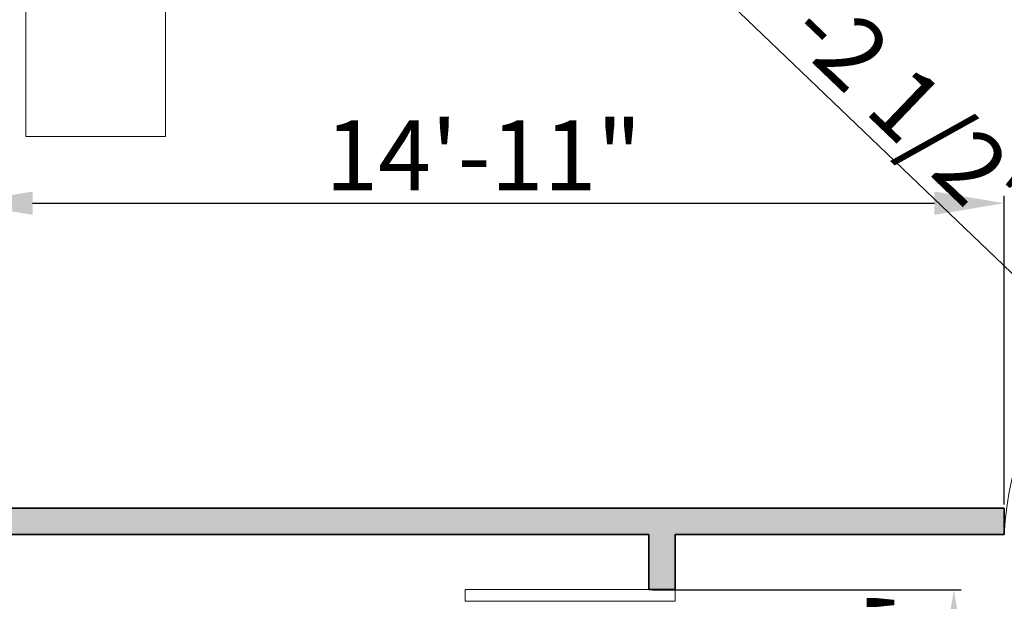
# Model space of a CAD drawing. Units: inches. Extents: x 2083 to 3317, y 1141 to 2115.
# Tile 93 of 256: x 2246 to 2415, y 1794 to 1894. Entities that reach past the tile are written whole.
import ezdxf

# ---------------------------------------------------------------- set-up
doc = ezdxf.new("R2010")
doc.units = ezdxf.units.IN
for name, color, linetype, lineweight in [('A-ANNO-DIMS', 2, 'Continuous', 18), ('A-DOOR', 4, 'Continuous', 18), ('A-FURN', 8, 'Continuous', 18), ('A-WALL', 7, 'Continuous', 35)]:
    doc.layers.add(name, color=color, linetype=linetype, lineweight=lineweight)
doc.layers.add('A-WALL-PATT', color=251, linetype='Continuous', lineweight=13, true_color=0x636466)
doc.styles.get("Standard").update_dxf_attribs({"font": 'arial.ttf'})
doc.dimstyles.new('ISO-25', dxfattribs={"dimtxt": 12, "dimasz": 12, "dimexe": 1.25, "dimexo": 0.625, "dimtad": 1, "dimlunit": 3, "dimtxsty": 'Standard', "dimcen": 2.5, "dimadec": 0, "dimazin": 0, "dimtfac": 1, "dimtmove": 0, "dimatfit": 3, "dimfxl": 1, "dimarcsym": 0})

# ---------------------------------------------------------------- blocks, each defined once
blk = doc.blocks.new('*D53')
at = {"layer": 'A-ANNO-DIMS', "color": 0, "lineweight": -2, "transparency": 16777216}
for p, q in [((2235.96, 1810.64), (2235.96, 1863.61)), ((2247.96, 1862.36), (2402.72, 1862.36)), ((2414.72, 1810.64), (2414.72, 1863.61))]:
    blk.add_line(p, q, dxfattribs=at)
at = {"layer": 'A-ANNO-DIMS', "color": 0, "transparency": 16777216}
for points in [[(2247.96, 1864.36), (2247.96, 1860.36), (2235.96, 1862.36)], [(2402.72, 1864.36), (2402.72, 1860.36), (2414.72, 1862.36)]]:
    blk.add_solid(points, dxfattribs=at)
at = {"layer": 'Defpoints', "color": 0, "transparency": 16777216}
for p in [(2414.72, 1862.36), (2235.96, 1810.01), (2414.72, 1810.01)]:
    blk.add_point(p, dxfattribs=at)
at = {"layer": 'A-ANNO-DIMS', "color": 0, "transparency": 16777216, "insert": (2325.34, 1869.01), "char_height": 12, "attachment_point": 5}
blk.add_mtext('14\'-11"', dxfattribs=at)
blk = doc.blocks.new('*D56')
at = {"layer": 'A-ANNO-DIMS', "color": 0, "lineweight": -2, "transparency": 16777216}
for p, q in [((2354.33, 1796.05), (2407.31, 1796.05)), ((2406.06, 1784.05), (2406.06, 1772.05)), ((2354.33, 1760.05), (2407.31, 1760.05))]:
    blk.add_line(p, q, dxfattribs=at)
at = {"layer": 'A-ANNO-DIMS', "color": 0, "transparency": 16777216}
for points in [[(2404.06, 1784.05), (2408.06, 1784.05), (2406.06, 1796.05)], [(2404.06, 1772.05), (2408.06, 1772.05), (2406.06, 1760.05)]]:
    blk.add_solid(points, dxfattribs=at)
at = {"layer": 'Defpoints', "color": 0, "transparency": 16777216}
for p in [(2353.71, 1796.05), (2353.71, 1760.05), (2406.06, 1760.05)]:
    blk.add_point(p, dxfattribs=at)
at = {"layer": 'A-ANNO-DIMS', "color": 0, "transparency": 16777216, "insert": (2399.3, 1778.05), "char_height": 12, "attachment_point": 5, "rotation": 90}
blk.add_mtext('3\'-0"', dxfattribs=at)
blk = doc.blocks.new('*D68')
at = {"layer": 'A-ANNO-DIMS', "color": 0, "lineweight": -2, "transparency": 16777216}
for p, q in [((2358.93, 1905.02), (2420.01, 1846.48)), ((2465.03, 1803.34), (2428.67, 1838.18))]:
    blk.add_line(p, q, dxfattribs=at)
at = {"layer": 'A-ANNO-DIMS', "color": 0, "transparency": 16777216}
blk.add_solid([(2421.39, 1847.93), (2418.62, 1845.04), (2428.67, 1838.18)], dxfattribs=at)
at = {"layer": 'Defpoints', "color": 0, "transparency": 16777216}
for p in [(2428.67, 1838.18), (2465.03, 1803.34)]:
    blk.add_point(p, dxfattribs=at)
at = {"layer": 'A-ANNO-DIMS', "color": 0, "transparency": 16777216, "insert": (2389.86, 1884.83), "char_height": 12, "attachment_point": 5, "rotation": 316.2184}
blk.add_mtext('R4\'-2 1/2"', dxfattribs=at)

msp = doc.modelspace()

# ---------------------------------------------------------------- hatches: boundary and pattern name
at = {"layer": 'A-WALL-PATT'}
h = msp.add_hatch(color=256, dxfattribs=at)
h.dxf.hatch_style = 1
h.paths.add_polyline_path([(3126.96, 2020.761), (2748.96, 2020.761), (2604.96, 2020.761), (2226.96, 2020.761), (2226.96, 1702.761), (2466.96, 1702.761), (2466.96, 1582.761), (2418.96, 1582.761), (2418.96, 1477.761), (2226.96, 1477.761), (2226.96, 1263.261), (2544.96, 1263.261), (2544.96, 1411.761), (2604.96, 1411.761), (2685.96, 1411.761), (2685.96, 1420.761), (2604.96, 1420.761), (2604.96, 1573.761), (2604.96, 1702.761), (2604.96, 2011.761), (2748.96, 2011.761), (2748.96, 1702.761), (2862.96, 1702.761), (2862.96, 1621.761), (2871.96, 1621.761), (2871.96, 1702.761), (2883.96, 1702.761), (2883.96, 1706.939, -0.0264593), (2883.96, 1711.761), (2757.96, 1711.761), (2757.96, 1807.761), (2787.96, 1807.761), (2787.96, 1812.261), (2757.96, 1812.261), (2757.96, 2011.761), (2877.96, 2011.761), (2877.96, 1812.261), (2847.96, 1812.261), (2847.96, 1807.761), (2889.836, 1807.761), (2889.836, 1812.261), (2882.46, 1812.261), (2882.46, 2011.761), (3117.96, 2011.761), (3117.96, 1812.261), (2937.836, 1812.261), (2937.836, 1807.761), (2995.71, 1807.761), (2995.71, 1796.118), (3000.21, 1796.118), (3000.21, 1807.761), (3117.96, 1807.761), (3117.96, 1711.761), (3000.21, 1711.761), (3000.21, 1760.118), (2998.573, 1760.118, -0.020711), (2995.71, 1760.118), (2995.71, 1711.761), (2931.96, 1711.761), (2931.96, 1702.761), (3126.96, 1702.761)])
h.paths.add_polyline_path([(2471.46, 2011.761), (2471.46, 1810.011), (2462.717, 1810.011), (2462.717, 1805.511), (2505.96, 1805.511), (2505.96, 1810.011), (2475.96, 1810.011), (2475.96, 2011.761), (2595.96, 2011.761), (2595.96, 1810.011), (2565.96, 1810.011), (2565.96, 1805.511), (2595.96, 1805.511), (2595.96, 1711.761), (2235.96, 1711.761), (2235.96, 1805.511), (2353.71, 1805.511), (2353.71, 1796.054), (2358.21, 1796.054), (2358.21, 1805.511), (2414.717, 1805.511), (2414.717, 1810.011), (2235.96, 1810.011), (2235.96, 2011.761)], flags=16)
h.paths.add_polyline_path([(2270.205, 1994.61), (2270.205, 1970.61), (2246.205, 1970.61), (2246.205, 1994.61)], flags=0)
edge = h.paths.add_edge_path(flags=0)
edge.add_ellipse((2332.027, 1899.798), major_axis=(-3.043, 3.043), ratio=0.1682525, start_angle=-161.33217, end_angle=-156.30711, ccw=False)
edge.add_ellipse((2333.082, 1898.744), major_axis=(-1.055, 1.055), ratio=0.4535321, start_angle=-123.37102, end_angle=-94.15911)
edge = h.paths.add_edge_path(flags=0)
edge.add_ellipse((2332.027, 1968.876), major_axis=(3.043, 3.043), ratio=0.1682525, start_angle=18.66783, end_angle=23.69289)
edge.add_spline(control_points=[(2332.926, 1970.691), (2332.227, 1970.336), (2330.894, 1969.659), (2328.413, 1970.932), (2327.204, 1967.749), (2324.71, 1969.956), (2322.533, 1967.012), (2320.013, 1971.296), (2317.68, 1968.158), (2316.041, 1967.102), (2315.427, 1966.81)], knot_values=[0, 0, 0, 0, 2.2670587, 4.3245589, 6.6855835, 8.8786411, 11.121502, 14.300359, 17.7552837, 19.732645, 19.732645, 19.732645, 19.732645], degree=3, periodic=0)
edge.add_ellipse((2332.027, 1968.876), major_axis=(3.043, 3.043), ratio=0.1682525, start_angle=18.66783, end_angle=23.69289, ccw=False)
edge.add_ellipse((2333.082, 1969.931), major_axis=(1.055, 1.055), ratio=0.4535321, start_angle=56.62898, end_angle=85.84089, ccw=False)
edge = h.paths.add_edge_path(flags=0)
edge.add_spline(control_points=[(2296.428, 1967.988), (2293.628, 1965.336), (2287.704, 1959.727), (2299.744, 1949.996), (2294.533, 1935.669), (2290.573, 1920.604), (2293.394, 1909.974), (2296.185, 1904.967)], knot_values=[0.0991853, 0.0991853, 0.0991853, 0.0991853, 0.3453009, 0.6198217, 0.9826526, 1.3860932, 1.8105546, 1.8105546, 1.8105546, 1.8105546], degree=3, periodic=0)
edge.add_spline(control_points=[(2296.185, 1904.967), (2297.384, 1902.619), (2298.001, 1901.949), (2298.553, 1901.468)], knot_values=[0.0062457, 0.0062457, 0.0062457, 0.0062457, 0.0554759, 0.0554759, 0.0554759, 0.0554759], degree=3, periodic=0)
edge.add_spline(control_points=[(2298.553, 1901.468), (2297.259, 1900.923), (2295.225, 1900.232), (2293.06, 1900.614), (2292.101, 1900.788), (2292.09, 1900.791)], knot_values=[0.3128349, 0.3128349, 0.3128349, 0.3128349, 0.4017797, 0.4749867, 0.4759027, 0.4759027, 0.4759027, 0.4759027], degree=3, periodic=0)
edge.add_arc((2292.794, 1904.664), 3.937, 215.4209, 259.69818, ccw=False)
edge.add_spline(control_points=[(2289.585, 1902.382), (2289.477, 1902.535), (2289.368, 1902.688), (2289.261, 1902.841)], knot_values=[0.1028719, 0.1028719, 0.1028719, 0.1028719, 0.1168958, 0.1168958, 0.1168958, 0.1168958], degree=3, periodic=0)
edge.add_spline(control_points=[(2289.261, 1902.841), (2288.687, 1902.55), (2287.64, 1902.02), (2285.881, 1901.874), (2283.853, 1901.504), (2281.72, 1899.711), (2278.467, 1899.493), (2276.157, 1901.883), (2272.259, 1899.804), (2267.778, 1901.843), (2262.244, 1900.184), (2257.415, 1901.782), (2254.318, 1900.726), (2253.178, 1900.337)], knot_values=[0, 0, 0, 0, 1.9079767, 3.4771759, 5.261074, 7.9728515, 11.6802485, 13.7179214, 16.9395917, 22.789562, 27.5025027, 33.5952153, 37.1456181, 37.1456181, 37.1456181, 37.1456181], degree=3, periodic=0)
edge.add_line((2253.178, 1900.337), (2250.244, 1902.841))
edge.add_line((2250.244, 1902.841), (2250.244, 1965.833))
edge.add_line((2250.244, 1965.833), (2253.178, 1968.337))
edge.add_spline(control_points=[(2253.178, 1968.337), (2254.318, 1967.948), (2257.415, 1966.892), (2262.244, 1968.49), (2267.778, 1966.831), (2271.527, 1968.537), (2273.876, 1967.828), (2274.207, 1967.728)], knot_values=[0, 0, 0, 0, 0.0901802, 0.2449351, 0.3646438, 0.5132331, 0.5378548, 0.5378548, 0.5378548, 0.5378548], degree=3, periodic=0)
edge.add_arc((2274.353, 1963.793), 3.937, 72.05113, 92.12795, ccw=False)
edge.add_arc((2281.297, 1985.23), 18.596, 252.05113, 288.56572)
edge.add_arc((2292.317, 1956.029), 12.646, 71.02679, 113.77822, ccw=False)
edge = h.paths.add_edge_path(flags=0)
edge.add_spline(control_points=[(2274.899, 1951.856), (2275.066, 1951.617), (2275.233, 1951.377), (2275.398, 1951.136)], knot_values=[1.4099157, 1.4099157, 1.4099157, 1.4099157, 1.4315903, 1.4315903, 1.4315903, 1.4315903], degree=3, periodic=0)
edge.add_spline(control_points=[(2275.398, 1951.136), (2275.792, 1950.562), (2276.179, 1949.984), (2276.546, 1949.397)], knot_values=[1.3582378, 1.3582378, 1.3582378, 1.3582378, 1.4099157, 1.4099157, 1.4099157, 1.4099157], degree=3, periodic=0)
edge.add_line((2276.546, 1949.397), (2277.437, 1947.862))
edge.add_spline(control_points=[(2277.437, 1947.862), (2276.304, 1945.673), (2274.64, 1942.427), (2274.632, 1938.094), (2272.799, 1930.852), (2274.356, 1943.897), (2275.948, 1947.923), (2276.546, 1949.397)], knot_values=[0.0056315, 0.0056315, 0.0056315, 0.0056315, 0.1860139, 0.2660015, 0.3570872, 0.5963902, 0.7397317, 0.7397317, 0.7397317, 0.7397317], degree=3, periodic=0)
edge.add_spline(control_points=[(2276.546, 1949.397), (2276.179, 1949.984), (2275.792, 1950.562), (2275.398, 1951.136)], knot_values=[1.3582378, 1.3582378, 1.3582378, 1.3582378, 1.4099157, 1.4099157, 1.4099157, 1.4099157], degree=3, periodic=0)
edge.add_spline(control_points=[(2275.398, 1951.136), (2274.943, 1950.08), (2274.208, 1948.025), (2273.935, 1944.851), (2272.469, 1937.627), (2273.466, 1945.696), (2274.701, 1951.059), (2274.899, 1951.856)], knot_values=[0.1043639, 0.1043639, 0.1043639, 0.1043639, 0.1896363, 0.2696239, 0.3607096, 0.6000126, 0.6446217, 0.6446217, 0.6446217, 0.6446217], degree=3, periodic=0)
h.paths.add_polyline_path([(2269.168, 1963.128, -0.3575267), (2268.171, 1960.976, -0.0925607), (2268.171, 1939.436, -0.3575267), (2269.168, 1937.285, -0.3575267), (2267.016, 1938.282, -0.1647847), (2254.686, 1938.282, -0.3575267), (2252.534, 1937.285, -0.3575267), (2253.531, 1939.436, -0.0925607), (2253.531, 1960.976, -0.3575267), (2252.534, 1963.128, -0.3575267), (2254.686, 1962.131, -0.1647847), (2267.016, 1962.131, -0.3575267)], flags=0)
h.paths.add_polyline_path([(2248.874, 1967.802), (2248.874, 1957.028), (2249.458, 1957.028), (2249.458, 1911.647), (2248.874, 1911.647), (2248.874, 1900.873), (2246.512, 1900.873, 0.1973271), (2244.15, 1902.457), (2244.15, 1966.218, 0.1973271), (2246.512, 1967.802)], flags=0)
h.paths.add_polyline_path([(2269.168, 1931.389, -0.3575267), (2268.171, 1929.238, -0.0925607), (2268.171, 1907.698, -0.3575267), (2269.168, 1905.547, -0.3575267), (2267.016, 1906.544, -0.1647847), (2254.686, 1906.544, -0.3575267), (2252.534, 1905.547, -0.3575267), (2253.531, 1907.698, -0.0925607), (2253.531, 1929.238, -0.3575267), (2252.534, 1931.389, -0.3575267), (2254.686, 1930.392, -0.1647847), (2267.016, 1930.392, -0.3575267)], flags=0)
edge = h.paths.add_edge_path(flags=0)
edge.add_spline(control_points=[(2276.197, 1906.724), (2276.168, 1909.029), (2276.114, 1913.372), (2270.598, 1924.925), (2273.905, 1919.013), (2275.922, 1916.262), (2275.475, 1912.402), (2277.258, 1910.381), (2276.696, 1908.225), (2276.646, 1906.813), (2276.618, 1906.008)], knot_values=[0, 0, 0, 0, 8.6102597, 16.2212739, 18.8430575, 23.8048978, 27.4408283, 29.3561016, 31.2034776, 33.6506866, 33.6506866, 33.6506866, 33.6506866], degree=3, periodic=0)
edge.add_spline(control_points=[(2276.618, 1906.008), (2276.623, 1905.624), (2276.498, 1904.629), (2275.442, 1903.855), (2274.937, 1903.08), (2274.859, 1902.841)], knot_values=[0.1564884, 0.1564884, 0.1564884, 0.1564884, 0.1843975, 0.2313765, 0.2505985, 0.2505985, 0.2505985, 0.2505985], degree=3, periodic=0)
edge.add_line((2274.859, 1902.841), (2276.506, 1902.841))
edge.add_spline(control_points=[(2276.506, 1902.841), (2276.788, 1903.085), (2277.665, 1904.125), (2278.25, 1904.341), (2277.654, 1908.527), (2278.156, 1906.228), (2278.1, 1905.286), (2278.847, 1904.069), (2277.857, 1903.415), (2277.874, 1902.991), (2277.904, 1902.841)], knot_values=[0.0595743, 0.0595743, 0.0595743, 0.0595743, 0.0807529, 0.1037415, 0.1697201, 0.1760361, 0.2071372, 0.2404744, 0.2623409, 0.2736605, 0.2736605, 0.2736605, 0.2736605], degree=3, periodic=0)
edge.add_line((2277.904, 1902.841), (2280.03, 1902.841))
edge.add_spline(control_points=[(2280.03, 1902.841), (2279.888, 1903.088), (2279.499, 1903.982), (2280.152, 1905.939), (2278.104, 1909.658), (2279.762, 1907.185), (2280.328, 1904.875), (2280.485, 1903.49), (2281.463, 1903.249), (2281.758, 1902.936), (2281.834, 1902.841)], knot_values=[0.013856, 0.013856, 0.013856, 0.013856, 0.0348738, 0.0888667, 0.1078792, 0.1267378, 0.158714, 0.1937575, 0.2174868, 0.2267221, 0.2267221, 0.2267221, 0.2267221], degree=3, periodic=0)
edge.add_spline(control_points=[(2281.834, 1902.841), (2281.788, 1902.827), (2281.647, 1902.783), (2281.396, 1902.859), (2281.088, 1902.985), (2280.721, 1903.061), (2280.333, 1903.026), (2280.125, 1902.899), (2280.03, 1902.841)], knot_values=[0, 0, 0, 0, 0.1441304, 0.435517, 0.7492759, 1.1530457, 1.5483707, 1.878348, 1.878348, 1.878348, 1.878348], degree=3, periodic=0)
edge.add_line((2280.03, 1902.841), (2277.904, 1902.841))
edge.add_spline(control_points=[(2277.904, 1902.841), (2277.893, 1902.796), (2277.865, 1902.68), (2277.607, 1902.687), (2277.274, 1902.801), (2276.838, 1902.62), (2276.584, 1902.789), (2276.506, 1902.841)], knot_values=[0, 0, 0, 0, 0.1271885, 0.3261988, 0.6280094, 1.2435704, 1.5153306, 1.5153306, 1.5153306, 1.5153306], degree=3, periodic=0)
edge.add_line((2276.506, 1902.841), (2274.859, 1902.841))
edge.add_spline(control_points=[(2274.859, 1902.841), (2274.814, 1902.899), (2274.725, 1903.013), (2274.493, 1903.119), (2274.244, 1902.961), (2273.937, 1903.185), (2273.614, 1902.983), (2273.408, 1902.883), (2273.322, 1902.841)], knot_values=[0, 0, 0, 0, 0.2184302, 0.4369566, 0.6879766, 0.9903786, 1.3983955, 1.6918498, 1.6918498, 1.6918498, 1.6918498], degree=3, periodic=0)
edge.add_spline(control_points=[(2273.322, 1902.841), (2273.617, 1903.446), (2274.274, 1904.538), (2276.027, 1904.574), (2276.207, 1906.584), (2276.197, 1906.724)], knot_values=[0.0122268, 0.0122268, 0.0122268, 0.0122268, 0.0594721, 0.1062177, 0.134458, 0.134458, 0.134458, 0.134458], degree=3, periodic=0)
h.paths.add_polyline_path([(2270.776, 1897.79), (2270.776, 1873.79), (2246.776, 1873.79), (2246.776, 1897.79)], flags=0)
h.paths.add_polyline_path([(2353.71, 1760.005), (2353.71, 1760.054), (2358.21, 1760.054, -0.033729)], flags=0)
h.paths.add_polyline_path([(2321.819, 1737.529), (2341.995, 1737.529, -0.4142136), (2343.203, 1736.321), (2343.203, 1721.021, -0.4142136), (2341.995, 1719.813), (2321.819, 1719.813, -0.4142136), (2320.611, 1721.021), (2320.611, 1736.321, -0.4142136)], flags=0)
h.paths.add_polyline_path([(2324.235, 1736.321), (2339.579, 1736.321, -0.4142136), (2341.995, 1733.905), (2341.995, 1725.45, -0.4142136), (2339.579, 1723.034), (2333.681, 1723.034), (2333.845, 1722.045, -0.8706461), (2335.425, 1721.826, -0.767327), (2333.923, 1721.423), (2331.291, 1721.423, -0.767327), (2329.788, 1721.826, -0.8706461), (2331.368, 1722.045), (2331.533, 1723.034), (2324.235, 1723.034, -0.4142136), (2321.819, 1725.45), (2321.819, 1733.905, -0.4142136)], flags=0)
h.paths.add_polyline_path([(2570.484, 1928.615), (2589.684, 1928.615), (2590.169, 1928.615), (2590.169, 1904.993), (2570.484, 1904.993)], flags=0)
h.paths.add_polyline_path([(2574.447, 1927.264, -1), (2572.829, 1927.264, -1)], flags=0)
h.paths.add_polyline_path([(2573.09, 1926.941), (2573.925, 1927.776), (2574.148, 1927.553), (2573.313, 1926.718)], flags=0)
h.paths.add_polyline_path([(2578.779, 1919.73, -1), (2571.592, 1919.73, -1)], flags=0)
h.paths.add_polyline_path([(2578.385, 1919.73, -1), (2571.985, 1919.73, -1)], flags=0)
h.paths.add_polyline_path([(2331.596, 1729.476, -1), (2333.618, 1729.476, -1)], flags=0)
h.paths.add_polyline_path([(2578.034, 1927.264, -1), (2576.416, 1927.264, -1)], flags=0)
h.paths.add_polyline_path([(2576.689, 1927.531), (2576.912, 1927.754), (2577.747, 1926.919), (2577.524, 1926.696)], flags=0)
h.paths.add_polyline_path([(2578.139, 1909.86, -1), (2572.232, 1909.86, -1)], flags=0)
h.paths.add_polyline_path([(2577.745, 1909.86, -1), (2572.625, 1909.86, -1)], flags=0)
h.paths.add_polyline_path([(2583.798, 1927.264, -1), (2582.179, 1927.264, -1)], flags=0)
h.paths.add_polyline_path([(2582.719, 1927.754), (2583.554, 1926.919), (2583.331, 1926.696), (2582.496, 1927.531)], flags=0)
h.paths.add_polyline_path([(2582.496, 1927.531), (2582.719, 1927.754), (2583.554, 1926.919), (2583.331, 1926.696)], flags=0)
h.paths.add_polyline_path([(2587.739, 1920.53, -1), (2581.832, 1920.53, -1)], flags=0)
h.paths.add_polyline_path([(2587.345, 1920.53, -1), (2582.225, 1920.53, -1)], flags=0)
h.paths.add_polyline_path([(2587.385, 1927.264, -1), (2585.766, 1927.264, -1)], flags=0)
h.paths.add_polyline_path([(2586.082, 1926.98), (2586.917, 1927.815), (2587.14, 1927.593), (2586.305, 1926.758)], flags=0)
h.paths.add_polyline_path([(2588.379, 1910.66, -1), (2581.192, 1910.66, -1)], flags=0)
h.paths.add_polyline_path([(2587.985, 1910.66, -1), (2581.585, 1910.66, -1)], flags=0)
h.paths.add_polyline_path([(2417.168, 1729.478), (2437.344, 1729.478, -0.4142136), (2438.552, 1728.27), (2438.552, 1712.969, -0.4142136), (2437.344, 1711.761), (2417.168, 1711.761, -0.4142136), (2415.96, 1712.969), (2415.96, 1728.27, -0.4142136)], flags=0)
h.paths.add_polyline_path([(2419.584, 1728.27), (2434.928, 1728.27, -0.4142136), (2437.344, 1725.854), (2437.344, 1717.398, -0.4142136), (2434.928, 1714.983), (2429.029, 1714.983), (2429.194, 1713.994, -0.8706461), (2430.774, 1713.775, -0.767327), (2429.271, 1713.372), (2426.64, 1713.372, -0.767327), (2425.137, 1713.775, -0.8706461), (2426.717, 1713.994), (2426.882, 1714.983), (2419.584, 1714.983, -0.4142136), (2417.168, 1717.398), (2417.168, 1725.854, -0.4142136)], flags=0)
h.paths.add_polyline_path([(2419.584, 1728.27), (2434.928, 1728.27, -0.4142136), (2437.344, 1725.854), (2437.344, 1717.398, -0.4142136), (2434.928, 1714.983), (2429.029, 1714.983), (2428.358, 1719.009), (2427.553, 1719.009), (2426.882, 1714.983), (2419.584, 1714.983, -0.4142136), (2417.168, 1717.398), (2417.168, 1725.854, -0.4142136)], flags=0)
h.paths.add_polyline_path([(2426.944, 1721.425, -1), (2428.967, 1721.425, -1)], flags=0)
h.paths.add_polyline_path([(2475.96, 1702.761), (2595.96, 1702.761), (2595.96, 1582.761), (2475.96, 1582.761)], flags=16)
h.paths.add_polyline_path([(2427.96, 1573.761), (2595.96, 1573.761), (2595.96, 1468.761), (2595.96, 1420.761), (2384.46, 1420.761), (2384.46, 1468.761), (2427.96, 1468.761)], flags=16)
h.paths.add_polyline_path([(2379.96, 1468.761), (2379.96, 1420.761), (2235.96, 1420.761), (2235.96, 1468.761)], flags=16)
h.paths.add_polyline_path([(2317.816, 1466.696), (2337.992, 1466.696, -0.4142136), (2339.2, 1465.488), (2339.2, 1450.187, -0.4142136), (2337.992, 1448.979), (2317.816, 1448.979, -0.4142136), (2316.608, 1450.187), (2316.608, 1465.488, -0.4142136)], flags=0)
h.paths.add_polyline_path([(2320.232, 1465.488), (2335.576, 1465.488, -0.4142136), (2337.992, 1463.072), (2337.992, 1454.616, -0.4142136), (2335.576, 1452.2), (2329.677, 1452.2), (2329.842, 1451.212, -0.8706461), (2331.422, 1450.992, -0.767327), (2329.92, 1450.59), (2327.288, 1450.59, -0.767327), (2325.785, 1450.992, -0.8706461), (2327.365, 1451.212), (2327.53, 1452.2), (2320.232, 1452.2, -0.4142136), (2317.816, 1454.616), (2317.816, 1463.072, -0.4142136)], flags=0)
h.paths.add_polyline_path([(2320.232, 1465.488), (2335.576, 1465.488, -0.4142136), (2337.992, 1463.072), (2337.992, 1454.616, -0.4142136), (2335.576, 1452.2), (2329.677, 1452.2), (2329.006, 1456.227), (2328.201, 1456.227), (2327.53, 1452.2), (2320.232, 1452.2, -0.4142136), (2317.816, 1454.616), (2317.816, 1463.072, -0.4142136)], flags=0)
h.paths.add_polyline_path([(2327.593, 1458.643, -1), (2329.615, 1458.643, -1)], flags=0)
h.paths.add_polyline_path([(2244.412, 1433.34), (2241.921, 1433.34, -0.4142136), (2240.018, 1435.244), (2240.018, 1440.953, -0.4142105), (2241.921, 1442.856), (2244.412, 1442.856, -1.9764724)], flags=0)
h.paths.add_polyline_path([(2245.357, 1434.398, -0.4142136), (2245.357, 1441.799, -2.1440985)], flags=0)
h.paths.add_polyline_path([(2535.96, 1416.261), (2535.96, 1272.261), (2235.96, 1272.261), (2235.96, 1416.261)], flags=16)
h.paths.add_polyline_path([(2260.12, 1384.293), (2260.12, 1362.039), (2237.865, 1362.039), (2237.865, 1384.293)], flags=0)
edge = h.paths.add_edge_path(flags=0)
edge.add_line((2318.252, 1362.093), (2318.146, 1362.001))
edge.add_ellipse((2317.445, 1360.431), major_axis=(2.822, 2.822), ratio=0.1682525, start_angle=18.66783, end_angle=20.94813, ccw=False)
edge.add_ellipse((2318.423, 1361.409), major_axis=(0.978, 0.978), ratio=0.4535321, start_angle=56.62898, end_angle=70.2262, ccw=False)
edge = h.paths.add_edge_path(flags=0)
edge.add_line((2319.107, 1295.571), (2319.015, 1295.677))
edge.add_ellipse((2317.445, 1296.378), major_axis=(-2.822, 2.822), ratio=0.1682525, start_angle=-161.33217, end_angle=-159.05187, ccw=False)
edge.add_ellipse((2318.423, 1295.4), major_axis=(-0.978, 0.978), ratio=0.4535321, start_angle=-123.37102, end_angle=-109.7738)
edge = h.paths.add_edge_path(flags=0)
edge.add_spline(control_points=[(2284.21, 1301.17), (2284.581, 1300.445), (2284.891, 1299.892), (2285.16, 1299.461)], knot_values=[0.0390658, 0.0390658, 0.0390658, 0.0390658, 0.0554759, 0.0554759, 0.0554759, 0.0554759], degree=3, periodic=0)
edge.add_line((2285.16, 1299.461), (2284.21, 1301.17))
edge = h.paths.add_edge_path(flags=0)
edge.add_line((2280.412, 1297.298), (2283.37, 1297.036))
edge.add_line((2283.37, 1297.036), (2286.406, 1297.926))
edge.add_spline(control_points=[(2286.406, 1297.926), (2285.305, 1297.463), (2284.345, 1297.129), (2283.37, 1297.036)], knot_values=[0.3943688, 0.3943688, 0.3943688, 0.3943688, 0.4759027, 0.4759027, 0.4759027, 0.4759027], degree=3, periodic=0)
edge.add_spline(control_points=[(2283.37, 1297.036), (2283.281, 1297.028), (2282.316, 1296.957), (2281.313, 1297.134), (2280.423, 1297.296), (2280.412, 1297.298)], knot_values=[0.3128349, 0.3128349, 0.3128349, 0.3128349, 0.3202458, 0.3934528, 0.3943688, 0.3943688, 0.3943688, 0.3943688], degree=3, periodic=0)
edge = h.paths.add_edge_path(flags=0)
edge.add_line((2284.436, 1359.607), (2280.446, 1355.328))
edge.add_line((2280.446, 1355.328), (2279.58, 1351.018))
edge.add_line((2279.58, 1351.018), (2282.413, 1346.58))
edge.add_spline(control_points=[(2282.413, 1346.58), (2283.153, 1345.589), (2284.253, 1344.029), (2284.801, 1342.387), (2284.935, 1341.806)], knot_values=[1.2400982, 1.2400982, 1.2400982, 1.2400982, 1.3328922, 1.3827123, 1.3827123, 1.3827123, 1.3827123], degree=3, periodic=0)
edge.add_spline(control_points=[(2284.935, 1341.806), (2285.319, 1340.141), (2285.233, 1338.409), (2284.91, 1336.654)], knot_values=[1.0974841, 1.0974841, 1.0974841, 1.0974841, 1.2400982, 1.2400982, 1.2400982, 1.2400982], degree=3, periodic=0)
edge.add_spline(control_points=[(2284.91, 1336.654), (2284.587, 1334.899), (2284.027, 1333.12), (2283.463, 1331.361)], knot_values=[0.9548699, 0.9548699, 0.9548699, 0.9548699, 1.0974841, 1.0974841, 1.0974841, 1.0974841], degree=3, periodic=0)
edge.add_line((2283.463, 1331.361), (2281.89, 1326.153))
edge.add_line((2281.89, 1326.153), (2280.756, 1321.056))
edge.add_line((2280.756, 1321.056), (2280.299, 1316.002))
edge.add_line((2280.299, 1316.002), (2280.716, 1310.95))
edge.add_line((2280.716, 1310.95), (2282.028, 1305.972))
edge.add_line((2282.028, 1305.972), (2284.21, 1301.17))
edge.add_spline(control_points=[(2284.21, 1301.17), (2283.341, 1302.73), (2282.612, 1304.336), (2282.028, 1305.972)], knot_values=[0.0991853, 0.0991853, 0.0991853, 0.0991853, 0.2417994, 0.2417994, 0.2417994, 0.2417994], degree=3, periodic=0)
edge.add_spline(control_points=[(2282.028, 1305.972), (2281.444, 1307.608), (2281.005, 1309.273), (2280.716, 1310.95)], knot_values=[0.2417994, 0.2417994, 0.2417994, 0.2417994, 0.3844135, 0.3844135, 0.3844135, 0.3844135], degree=3, periodic=0)
edge.add_spline(control_points=[(2280.716, 1310.95), (2280.433, 1312.588), (2280.289, 1314.277), (2280.299, 1315.962), (2280.299, 1316.002)], knot_values=[0.3844135, 0.3844135, 0.3844135, 0.3844135, 0.5236467, 0.5270276, 0.5270276, 0.5270276, 0.5270276], degree=3, periodic=0)
edge.add_spline(control_points=[(2280.299, 1316.002), (2280.312, 1317.687), (2280.478, 1319.368), (2280.756, 1321.056)], knot_values=[0.5270276, 0.5270276, 0.5270276, 0.5270276, 0.6696417, 0.6696417, 0.6696417, 0.6696417], degree=3, periodic=0)
edge.add_spline(control_points=[(2280.756, 1321.056), (2281.035, 1322.744), (2281.426, 1324.44), (2281.89, 1326.153)], knot_values=[0.6696417, 0.6696417, 0.6696417, 0.6696417, 0.8122558, 0.8122558, 0.8122558, 0.8122558], degree=3, periodic=0)
edge.add_spline(control_points=[(2281.89, 1326.153), (2282.264, 1327.533), (2282.788, 1329.262), (2283.353, 1331.018), (2283.463, 1331.361)], knot_values=[0.8122558, 0.8122558, 0.8122558, 0.8122558, 0.9270873, 0.9548699, 0.9548699, 0.9548699, 0.9548699], degree=3, periodic=0)
edge.add_line((2283.463, 1331.361), (2284.91, 1336.654))
edge.add_line((2284.91, 1336.654), (2284.935, 1341.806))
edge.add_line((2284.935, 1341.806), (2282.413, 1346.58))
edge.add_spline(control_points=[(2282.413, 1346.58), (2281.275, 1348.104), (2280.078, 1349.57), (2279.58, 1351.018)], knot_values=[1.3827123, 1.3827123, 1.3827123, 1.3827123, 1.5253264, 1.5253264, 1.5253264, 1.5253264], degree=3, periodic=0)
edge.add_spline(control_points=[(2279.58, 1351.018), (2279.443, 1351.415), (2279.136, 1352.857), (2279.735, 1354.29), (2280.446, 1355.328)], knot_values=[1.5253264, 1.5253264, 1.5253264, 1.5253264, 1.564439, 1.6679405, 1.6679405, 1.6679405, 1.6679405], degree=3, periodic=0)
edge.add_spline(control_points=[(2280.446, 1355.328), (2281.426, 1356.758), (2282.931, 1358.183), (2284.436, 1359.607)], knot_values=[1.6679405, 1.6679405, 1.6679405, 1.6679405, 1.8105546, 1.8105546, 1.8105546, 1.8105546], degree=3, periodic=0)
edge.add_arc((2280.623, 1348.518), 11.726, 71.02679, 113.77822)
edge.add_arc((2270.405, 1375.595), 17.244, 252.05113, 288.56572, ccw=False)
edge.add_arc((2263.966, 1355.718), 3.651, 72.05113, 92.12795)
edge.add_arc((2263.966, 1355.718), 3.651, 92.12795, 177.98513)
edge.add_spline(control_points=[(2260.318, 1355.846), (2260.26, 1354.221), (2260.551, 1350.187), (2262.999, 1346.766), (2264.473, 1344.649)], knot_values=[1.4315903, 1.4315903, 1.4315903, 1.4315903, 1.5641438, 1.7706953, 1.7706953, 1.7706953, 1.7706953], degree=3, periodic=0)
edge.add_line((2264.473, 1344.649), (2264.936, 1343.983))
edge.add_spline(control_points=[(2263.801, 1340.248), (2263.843, 1340.514), (2264.067, 1341.756), (2264.513, 1343.002), (2264.935, 1343.981)], knot_values=[0.5365702, 0.5365702, 0.5365702, 0.5365702, 0.5593494, 0.6446217, 0.6446217, 0.6446217, 0.6446217], degree=3, periodic=0)
edge.add_spline(control_points=[(2264.935, 1343.981), (2265.118, 1343.715), (2265.299, 1343.448), (2265.477, 1343.179)], knot_values=[1.3840767, 1.3840767, 1.3840767, 1.3840767, 1.4099157, 1.4099157, 1.4099157, 1.4099157], degree=3, periodic=0)
edge.add_spline(control_points=[(2265.477, 1343.179), (2265.655, 1342.911), (2265.829, 1342.641), (2265.999, 1342.369)], knot_values=[1.3582378, 1.3582378, 1.3582378, 1.3582378, 1.3840767, 1.3840767, 1.3840767, 1.3840767], degree=3, periodic=0)
edge.add_line((2265.999, 1342.369), (2266.826, 1340.946))
edge.add_spline(control_points=[(2266.826, 1340.946), (2268.894, 1337.09), (2271.398, 1325.843), (2270.516, 1310.569), (2275.919, 1301.861), (2277.79, 1299.199)], knot_values=[0.1168958, 0.1168958, 0.1168958, 0.1168958, 0.4729873, 1.0509689, 1.3137934, 1.3137934, 1.3137934, 1.3137934], degree=3, periodic=0)
edge.add_spline(control_points=[(2277.79, 1299.199), (2277.839, 1299.128), (2277.889, 1299.057), (2277.94, 1298.987)], knot_values=[0.1098839, 0.1098839, 0.1098839, 0.1098839, 0.1168958, 0.1168958, 0.1168958, 0.1168958], degree=3, periodic=0)
edge.add_line((2277.94, 1298.987), (2277.789, 1299.199))
edge.add_spline(control_points=[(2277.789, 1299.199), (2277.257, 1298.929), (2276.286, 1298.438), (2275.039, 1298.334), (2274.383, 1298.239), (2274.215, 1298.209)], knot_values=[33.1218702, 33.1218702, 33.1218702, 33.1218702, 35.0290557, 36.5982549, 37.1448269, 37.1448269, 37.1448269, 37.1448269], degree=3, periodic=0)
edge.add_line((2274.215, 1298.209), (2273.073, 1297.893))
edge.add_spline(control_points=[(2273.073, 1297.893), (2272.323, 1297.58), (2271.039, 1296.511), (2269.248, 1296.226), (2268.423, 1296.375)], knot_values=[26.5325843, 26.5325843, 26.5325843, 26.5325843, 29.198919, 31.8391012, 31.8391012, 31.8391012, 31.8391012], degree=3, periodic=0)
edge.add_line((2268.423, 1296.375), (2263.879, 1297.458))
edge.add_spline(control_points=[(2263.879, 1297.458), (2263.556, 1297.359), (2261.86, 1296.839), (2260.239, 1297.282), (2258.933, 1297.516)], knot_values=[15.9195506, 15.9195506, 15.9195506, 15.9195506, 16.9395917, 21.2260675, 21.2260675, 21.2260675, 21.2260675], degree=3, periodic=0)
edge.add_line((2258.933, 1297.516), (2254.055, 1297.329))
edge.add_spline(control_points=[(2254.055, 1297.329), (2253.756, 1297.296), (2252.114, 1297.165), (2250.462, 1297.544), (2249.13, 1297.668)], knot_values=[5.3065169, 5.3065169, 5.3065169, 5.3065169, 6.2764352, 10.6130337, 10.6130337, 10.6130337, 10.6130337], degree=3, periodic=0)
edge.add_line((2249.13, 1297.668), (2244.332, 1296.878))
edge.add_line((2244.332, 1296.878), (2241.611, 1299.199))
edge.add_line((2241.611, 1299.199), (2241.611, 1357.609))
edge.add_line((2241.611, 1357.609), (2244.332, 1359.931))
edge.add_line((2244.332, 1359.931), (2252.729, 1359.543))
edge.add_spline(control_points=[(2252.729, 1359.543), (2252.871, 1359.546), (2253.306, 1359.548), (2253.74, 1359.514), (2254.032, 1359.482)], knot_values=[0.233291, 0.233291, 0.233291, 0.233291, 0.2449351, 0.2689274, 0.2689274, 0.2689274, 0.2689274], degree=3, periodic=0)
edge.add_line((2254.032, 1359.482), (2259.587, 1359.416))
edge.add_spline(control_points=[(2259.587, 1359.416), (2260.677, 1359.629), (2262.073, 1359.897), (2263.524, 1359.459), (2263.83, 1359.366)], knot_values=[0.4225164, 0.4225164, 0.4225164, 0.4225164, 0.5132331, 0.5378548, 0.5378548, 0.5378548, 0.5378548], degree=3, periodic=0)
edge.add_arc((2263.966, 1355.718), 3.651, 72.05113, 92.12795, ccw=False)
edge.add_arc((2270.405, 1375.595), 17.244, 252.05113, 288.56572)
edge.add_arc((2280.623, 1348.518), 11.726, 71.02679, 113.77822, ccw=False)
h.paths.add_polyline_path([(2240.341, 1359.435), (2240.341, 1349.444), (2240.882, 1349.444), (2240.882, 1307.365), (2240.341, 1307.365), (2240.341, 1297.374), (2238.15, 1297.374, 0.1973271), (2235.96, 1298.843), (2235.96, 1357.966, 0.1973271), (2238.15, 1359.435)], flags=0)
h.paths.add_polyline_path([(2259.158, 1355.101, -0.3575267), (2258.233, 1353.106, -0.0925607), (2258.233, 1333.133, -0.3575267), (2259.158, 1331.138, -0.3575267), (2257.163, 1332.062, -0.1647847), (2245.729, 1332.062, -0.3575267), (2243.735, 1331.138, -0.3575267), (2244.659, 1333.133, -0.0925607), (2244.659, 1353.106, -0.3575267), (2243.735, 1355.101, -0.3575267), (2245.729, 1354.176, -0.1647847), (2257.163, 1354.176, -0.3575267)], flags=0)
edge = h.paths.add_edge_path(flags=0)
edge.add_line((2265.999, 1342.369), (2266.826, 1340.946))
edge.add_line((2266.826, 1340.946), (2265.308, 1337.814))
edge.add_line((2265.308, 1337.814), (2264.358, 1334.653))
edge.add_line((2264.358, 1334.653), (2264.262, 1333.8))
edge.add_spline(control_points=[(2264.262, 1333.8), (2264.208, 1333.187), (2264.162, 1332.366), (2264.007, 1331.414), (2263.969, 1331.202)], knot_values=[0.4644442, 0.4644442, 0.4644442, 0.4644442, 0.5166905, 0.5316081, 0.5316081, 0.5316081, 0.5316081], degree=3, periodic=0)
edge.add_spline(control_points=[(2263.969, 1331.202), (2263.775, 1330.119), (2263.424, 1328.791), (2263.257, 1328.531), (2263.234, 1328.515)], knot_values=[0.3726816, 0.3726816, 0.3726816, 0.3726816, 0.4488497, 0.4644442, 0.4644442, 0.4644442, 0.4644442], degree=3, periodic=0)
edge.add_spline(control_points=[(2263.234, 1328.515), (2263.096, 1328.42), (2263.131, 1329.301), (2263.275, 1330.616)], knot_values=[0.2809191, 0.2809191, 0.2809191, 0.2809191, 0.3726816, 0.3726816, 0.3726816, 0.3726816], degree=3, periodic=0)
edge.add_spline(control_points=[(2263.275, 1330.616), (2263.419, 1331.93), (2263.672, 1333.677), (2263.97, 1335.315)], knot_values=[0.1891566, 0.1891566, 0.1891566, 0.1891566, 0.2809191, 0.2809191, 0.2809191, 0.2809191], degree=3, periodic=0)
edge.add_spline(control_points=[(2263.97, 1335.315), (2264.1, 1336.032), (2264.419, 1337.622), (2264.755, 1338.864), (2264.947, 1339.491)], knot_values=[0.097394, 0.097394, 0.097394, 0.097394, 0.1375775, 0.1891566, 0.1891566, 0.1891566, 0.1891566], degree=3, periodic=0)
edge.add_spline(control_points=[(2264.947, 1339.491), (2265.29, 1340.606), (2265.644, 1341.494), (2265.999, 1342.369)], knot_values=[0.0056315, 0.0056315, 0.0056315, 0.0056315, 0.097394, 0.097394, 0.097394, 0.097394], degree=3, periodic=0)
h.paths.add_polyline_path([(2259.158, 1325.671, -0.3575267), (2258.233, 1323.676, -0.0925607), (2258.233, 1303.703, -0.3575267), (2259.158, 1301.708, -0.3575267), (2257.163, 1302.633, -0.1647847), (2245.729, 1302.633, -0.3575267), (2243.735, 1301.708, -0.3575267), (2244.659, 1303.703, -0.0925607), (2244.659, 1323.676, -0.3575267), (2243.735, 1325.671, -0.3575267), (2245.729, 1324.747, -0.1647847), (2257.163, 1324.747, -0.3575267)], flags=0)
edge = h.paths.add_edge_path(flags=0)
edge.add_spline(control_points=[(2261.709, 1317.311), (2261.679, 1317.418), (2261.762, 1317.389), (2262.491, 1316.09), (2262.962, 1315.301)], knot_values=[14.9558607, 14.9558607, 14.9558607, 14.9558607, 16.2212739, 18.6948259, 18.6948259, 18.6948259, 18.6948259], degree=3, periodic=0)
edge.add_spline(control_points=[(2262.962, 1315.301), (2262.99, 1315.254), (2263.702, 1314.067), (2264.349, 1313.127), (2264.73, 1312.164)], knot_values=[18.6948259, 18.6948259, 18.6948259, 18.6948259, 18.8430575, 22.433791, 22.433791, 22.433791, 22.433791], degree=3, periodic=0)
edge.add_spline(control_points=[(2264.73, 1312.164), (2264.876, 1311.796), (2265.177, 1310.77), (2265.143, 1309.559), (2265.248, 1308.824)], knot_values=[22.433791, 22.433791, 22.433791, 22.433791, 23.8048978, 26.1727562, 26.1727562, 26.1727562, 26.1727562], degree=3, periodic=0)
edge.add_line((2265.248, 1308.824), (2265.851, 1307.172))
edge.add_spline(control_points=[(2265.851, 1307.172), (2266.065, 1306.822), (2266.384, 1306.332), (2266.424, 1305.781), (2266.42, 1305.611)], knot_values=[28.0625624, 28.0625624, 28.0625624, 28.0625624, 29.3561016, 29.9117214, 29.9117214, 29.9117214, 29.9117214], degree=3, periodic=0)
edge.add_spline(control_points=[(2266.42, 1305.611), (2266.416, 1305.433), (2266.394, 1305.25), (2266.365, 1305.066)], knot_values=[29.9117214, 29.9117214, 29.9117214, 29.9117214, 30.4978371, 30.4978371, 30.4978371, 30.4978371], degree=3, periodic=0)
edge.add_line((2266.365, 1305.066), (2266.066, 1302.136))
edge.add_spline(control_points=[(2266.066, 1302.136), (2266.071, 1301.78), (2265.998, 1301.2), (2265.663, 1300.759), (2265.509, 1300.586)], knot_values=[0.1564884, 0.1564884, 0.1564884, 0.1564884, 0.1843975, 0.2035434, 0.2035434, 0.2035434, 0.2035434], degree=3, periodic=0)
edge.add_line((2265.509, 1300.586), (2264.435, 1299.199))
edge.add_line((2264.435, 1299.199), (2265.962, 1299.199))
edge.add_line((2265.962, 1299.199), (2267.336, 1301.175))
edge.add_line((2267.336, 1301.175), (2267.312, 1301.986))
edge.add_spline(control_points=[(2267.312, 1301.986), (2267.261, 1302.862), (2267.16, 1303.737), (2267.271, 1303.326)], knot_values=[0.1262286, 0.1262286, 0.1262286, 0.1262286, 0.1666174, 0.1666174, 0.1666174, 0.1666174], degree=3, periodic=0)
edge.add_spline(control_points=[(2267.271, 1303.326), (2267.28, 1303.294), (2267.31, 1303.175), (2267.373, 1302.884), (2267.406, 1302.683), (2267.418, 1302.601)], knot_values=[0.1666174, 0.1666174, 0.1666174, 0.1666174, 0.1697201, 0.1760361, 0.1807647, 0.1807647, 0.1807647, 0.1807647], degree=3, periodic=0)
edge.add_spline(control_points=[(2267.744, 1300.988), (2267.688, 1301.151), (2267.481, 1301.657), (2267.484, 1302.145), (2267.418, 1302.601)], knot_values=[0.1807647, 0.1807647, 0.1807647, 0.1807647, 0.1937665, 0.2201389, 0.2201389, 0.2201389, 0.2201389], degree=3, periodic=0)
edge.add_line((2267.418, 1302.601), (2267.744, 1300.988))
edge.add_spline(control_points=[(2267.744, 1300.988), (2267.832, 1300.732), (2267.932, 1300.31), (2267.555, 1299.975), (2267.429, 1299.829)], knot_values=[0.2201389, 0.2201389, 0.2201389, 0.2201389, 0.2404744, 0.2548903, 0.2548903, 0.2548903, 0.2548903], degree=3, periodic=0)
edge.add_line((2267.429, 1299.829), (2267.258, 1299.199))
edge.add_line((2267.258, 1299.199), (2269.23, 1299.199))
edge.add_spline(control_points=[(2269.23, 1299.199), (2269.099, 1299.429), (2268.843, 1300.016), (2269.012, 1300.916), (2268.947, 1301.661)], knot_values=[0.013856, 0.013856, 0.013856, 0.013856, 0.0348738, 0.0670726, 0.0670726, 0.0670726, 0.0670726], degree=3, periodic=0)
edge.add_line((2268.947, 1301.661), (2268.432, 1303.603))
edge.add_spline(control_points=[(2268.432, 1303.603), (2268.176, 1304.192), (2267.596, 1305.251), (2268.041, 1304.623), (2268.251, 1304.282)], knot_values=[0.0901547, 0.0901547, 0.0901547, 0.0901547, 0.1078792, 0.1202891, 0.1202891, 0.1202891, 0.1202891], degree=3, periodic=0)
edge.add_spline(control_points=[(2268.251, 1304.282), (2268.361, 1304.105), (2269.058, 1302.918), (2269.383, 1301.59), (2269.521, 1300.776), (2269.575, 1300.556)], knot_values=[0.1202891, 0.1202891, 0.1202891, 0.1202891, 0.1267378, 0.158714, 0.1735056, 0.1735056, 0.1735056, 0.1735056], degree=3, periodic=0)
edge.add_line((2269.575, 1300.556), (2270.686, 1299.421))
edge.add_spline(control_points=[(2270.686, 1299.421), (2270.767, 1299.357), (2270.838, 1299.281), (2270.903, 1299.199)], knot_values=[0.2181597, 0.2181597, 0.2181597, 0.2181597, 0.2267221, 0.2267221, 0.2267221, 0.2267221], degree=3, periodic=0)
edge.add_line((2270.937, 1299.193), (2270.903, 1299.199))
edge.add_spline(control_points=[(2270.903, 1299.199), (2270.86, 1299.186), (2270.73, 1299.146), (2270.496, 1299.216), (2270.272, 1299.308), (2270.121, 1299.348), (2270.063, 1299.36)], knot_values=[0.939174, 0.939174, 0.939174, 0.939174, 1.0833044, 1.3746911, 1.6884499, 1.878348, 1.878348, 1.878348, 1.878348], degree=3, periodic=0)
edge.add_line((2270.063, 1299.36), (2269.23, 1299.199))
edge.add_line((2269.23, 1299.199), (2267.258, 1299.199))
edge.add_spline(control_points=[(2267.258, 1299.199), (2267.248, 1299.157), (2267.223, 1299.05), (2266.984, 1299.057), (2266.809, 1299.116), (2266.677, 1299.109), (2266.637, 1299.105)], knot_values=[0.7576653, 0.7576653, 0.7576653, 0.7576653, 0.8848538, 1.0838641, 1.3856747, 1.5153306, 1.5153306, 1.5153306, 1.5153306], degree=3, periodic=0)
edge.add_spline(control_points=[(2266.637, 1299.105), (2266.485, 1299.089), (2266.236, 1299.017), (2266.035, 1299.151), (2265.962, 1299.199)], knot_values=[0, 0, 0, 0, 0.4859051, 0.7576653, 0.7576653, 0.7576653, 0.7576653], degree=3, periodic=0)
edge.add_line((2265.962, 1299.199), (2264.435, 1299.199))
edge.add_line((2264.435, 1299.199), (2263.858, 1299.367))
edge.add_spline(control_points=[(2263.858, 1299.367), (2263.819, 1299.371), (2263.78, 1299.386), (2263.74, 1299.402)], knot_values=[0.8459249, 0.8459249, 0.8459249, 0.8459249, 0.9786272, 0.9786272, 0.9786272, 0.9786272], degree=3, periodic=0)
edge.add_line((2263.722, 1299.396), (2263.01, 1299.199))
edge.add_spline(control_points=[(2263.01, 1299.199), (2263.246, 1299.683), (2263.506, 1300.128), (2263.873, 1300.408)], knot_values=[0.0122268, 0.0122268, 0.0122268, 0.0122268, 0.0529705, 0.0529705, 0.0529705, 0.0529705], degree=3, periodic=0)
edge.add_spline(control_points=[(2263.873, 1300.408), (2263.932, 1300.453), (2264.084, 1300.553), (2264.255, 1300.624), (2264.36, 1300.665)], knot_values=[0.0529705, 0.0529705, 0.0529705, 0.0529705, 0.0594721, 0.0690861, 0.0690861, 0.0690861, 0.0690861], degree=3, periodic=0)
edge.add_line((2264.36, 1300.665), (2265.142, 1301.078))
edge.add_line((2265.142, 1301.078), (2265.676, 1302.8))
edge.add_line((2265.676, 1302.8), (2265.541, 1305.704))
edge.add_line((2265.541, 1305.704), (2264.803, 1309.328))
edge.add_line((2264.803, 1309.328), (2263.041, 1314.092))
edge.add_spline(control_points=[(2263.041, 1314.092), (2262.384, 1315.671), (2261.796, 1316.998), (2261.709, 1317.311)], knot_values=[11.2168955, 11.2168955, 11.2168955, 11.2168955, 14.9558607, 14.9558607, 14.9558607, 14.9558607], degree=3, periodic=0)
h.paths.add_polyline_path([(2871.96, 1416.261), (2895.91, 1416.261), (2895.91, 1420.761), (2871.96, 1420.761), (2871.96, 1501.761), (2862.96, 1501.761), (2862.96, 1420.761), (2805.96, 1420.761), (2805.96, 1411.761), (2862.96, 1411.761), (2862.96, 1263.261), (3126.96, 1263.261), (3126.96, 1411.761), (3126.96, 1486.761), (2943.96, 1486.761), (2943.96, 1477.761), (2967.86, 1477.761), (2967.86, 1420.761), (2943.91, 1420.761), (2943.91, 1416.261), (3117.96, 1416.261), (3117.96, 1420.761), (2972.36, 1420.761), (2972.36, 1477.761), (3117.96, 1477.761), (3117.96, 1420.761), (3117.96, 1272.261), (2871.96, 1272.261)], flags=0)
h.paths.add_polyline_path([(2457.126, 1485.943), (2527.603, 1485.943), (2527.603, 1537.636), (2457.126, 1537.636)], flags=8)
h.paths.add_polyline_path([(2481.005, 1609.982), (2590.766, 1609.982), (2590.766, 1682.003), (2481.005, 1682.003)], flags=8)
h.paths.add_polyline_path([(2483.085, 1729.127), (2553.562, 1729.127), (2553.562, 1780.82), (2483.085, 1780.82)], flags=8)

# ---------------------------------------------------------------- linework, layer by layer
at = {"layer": 'A-DOOR'}
for p, q in [((2358.21, 1796.054), (2322.21, 1796.054)), ((2322.21, 1796.054), (2322.21, 1794.054)), ((2358.21, 1794.054), (2358.21, 1796.054)), ((2322.21, 1794.054), (2358.21, 1794.054))]:
    msp.add_line(p, q, dxfattribs=at)
msp.add_arc((2465.03, 1803.336), 50.36, 94.91324, 177.52451, dxfattribs=at)
at = {"layer": 'A-FURN'}
msp.add_lwpolyline([(2270.776, 1897.79), (2270.776, 1873.79), (2246.776, 1873.79), (2246.776, 1897.79)], close=True, dxfattribs=at)
at = {"layer": 'A-WALL'}
for p, q in [((2235.96, 1810.011), (2414.717, 1810.011)), ((2414.717, 1810.011), (2414.717, 1805.511)), ((2235.96, 1805.511), (2353.71, 1805.511)), ((2353.71, 1805.511), (2353.71, 1796.054)), ((2358.21, 1805.511), (2358.21, 1796.054)), ((2358.21, 1805.511), (2414.717, 1805.511)), ((2353.71, 1796.054), (2358.21, 1796.054))]:
    msp.add_line(p, q, dxfattribs=at)

# ---------------------------------------------------------------- dimensions: what is measured, and where the dimension line sits
at = {"layer": 'A-ANNO-DIMS'}
dim = msp.add_radius_dim(center=(2465.03, 1803.336), mpoint=(2428.671, 1838.181), dimstyle='ISO-25', override={"dimdec": 1, "dimlfac": 1, "dimrnd": 0, "dimzin": 1, "dimdsep": 46, "dimlunit": 4, "dimfrac": 2}, dxfattribs=at)
dim.commit()
dim.dimension.update_dxf_attribs({"geometry": '*D68', "text_midpoint": (2389.863, 1884.833)})
dim = msp.add_linear_dim(base=(2414.717, 1862.361), p1=(2235.96, 1810.011), p2=(2414.717, 1810.011), dimstyle='ISO-25', override={"dimdec": 1, "dimlfac": 1, "dimrnd": 0, "dimzin": 1, "dimdsep": 46, "dimlunit": 4, "dimfrac": 2}, dxfattribs=at)
dim.commit()
dim.dimension.update_dxf_attribs({"geometry": '*D53', "text_midpoint": (2325.338, 1869.011)})
dim = msp.add_linear_dim(base=(2406.06, 1760.054), p1=(2353.71, 1796.054), p2=(2353.71, 1760.054), angle=270, dimstyle='ISO-25', override={"dimdec": 1, "dimlfac": 1, "dimrnd": 0, "dimzin": 1, "dimdsep": 46, "dimlunit": 4, "dimfrac": 2}, dxfattribs=at)
dim.commit()
dim.dimension.update_dxf_attribs({"geometry": '*D56', "text_midpoint": (2399.304, 1778.054)})

doc.saveas('drawing.dxf')
